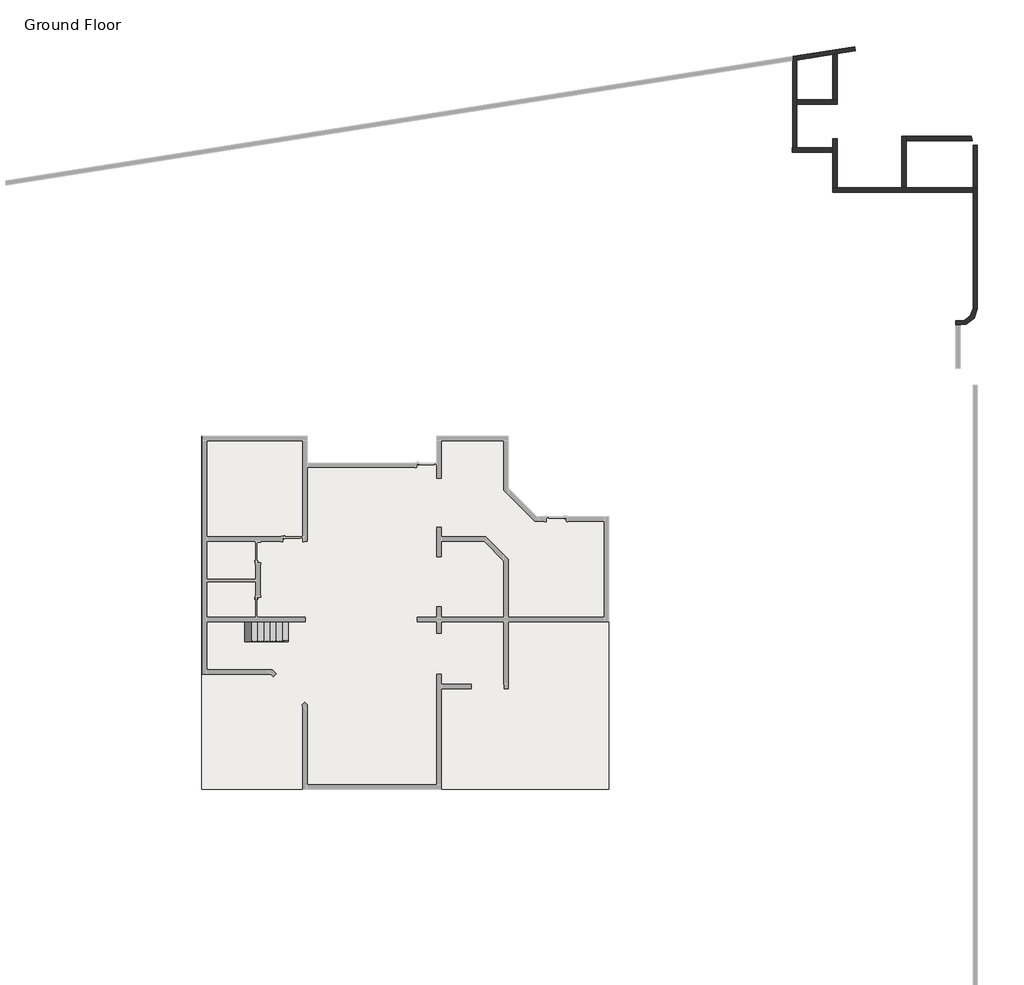
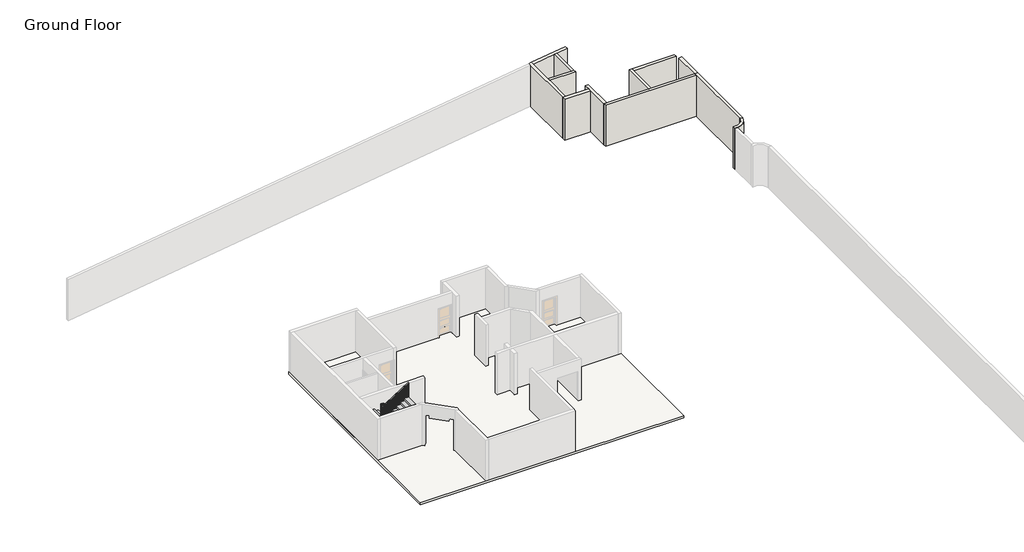
# One storey, part 2 of 2: 12 walls, 1 railing, 1 slab, 1 stair flight.
"""IFC4 building model written with IfcOpenShell, lengths in millimetres."""

from ifc_helpers import new_model, si_unit, point, frame, frame_2d, origin, origin_with_axes, place, context, project, spatial, polyline, circle_curve, trimmed, segment, composite_curve, outline, extrude, faceted_brep, element, save
from ifc_brep_helpers import plane_surface, cylinder_surface, revolved_surface, advanced_brep

model = new_model("IFC4")

# Units and contexts
model_context = context("Model", 3, world=origin())
ifc_project = project(units=[si_unit("LENGTHUNIT", "METRE", prefix="MILLI")], contexts=[model_context])

# Site, building, storey
site = spatial("IfcSite", under=ifc_project)
building = spatial("IfcBuilding", under=site)
storey = spatial("IfcBuildingStorey", under=building, Name="Ground Floor", Elevation=0.0)

# Railing
placement = place(None, origin())
element("IfcRailing", 1, ObjectType="Handrail - Rectangular", at=placement, inside=storey, context=model_context, shape_type="SolidModel", body=[
    faceted_brep([(-22136.7199287, -1918.1666371, 1093.6941176), (-22136.7199287, -1918.1666371, 1033.3090189), (-22136.7199287, -1867.3666371, 1033.3090189), (-22136.7199287, -1867.3666371, 1093.6941176), (-24850.5453762, -1918.1666371, 2837.6672398), (-24901.3453762, -1918.1666371, 2809.9275106), (-24901.3453762, -1867.3666371, 2809.9275106), (-24850.5453762, -1867.3666371, 2837.6672398), (-24926.7453762, -1994.3666371, 2835.8352941), (-24926.7453762, -1994.3666371, 2886.6352941), (-24926.7453762, -2196.4192808, 2886.6352941), (-24926.7453762, -2247.2192808, 2835.8352941), (-24977.5453762, -1994.3666371, 2835.8352941), (-24977.5453762, -2247.2192808, 2835.8352941), (-24977.5453762, -1994.3666371, 2886.6352941), (-24977.5453762, -2196.4192808, 2886.6352941), (-23259.8703762, -2272.6192808, 4141.6941176), (-23259.8703762, -2323.4192808, 4141.6941176), (-23259.8703762, -2323.4192808, 4081.2333039), (-23259.8703762, -2272.6192808, 4081.2333039), (-24835.5761466, -2272.6192808, 3064.3072269), (-24850.5453762, -2272.6192808, 3115.1072269), (-24835.5761466, -2323.4192808, 3064.3072269), (-24850.5453762, -2323.4192808, 3115.1072269), (-24850.5453762, -1918.1666371, 2886.6352941), (-24901.3453762, -1918.1666371, 2835.8352941), (-24901.3453762, -1867.3666371, 2835.8352941), (-24850.5453762, -1867.3666371, 2886.6352941), (-24926.7453762, -1918.1666371, 2886.6352941), (-24926.7453762, -1918.1666371, 2835.8352941), (-24977.5453762, -1867.3666371, 2835.8352941), (-24977.5453762, -1867.3666371, 2886.6352941), (-24926.7453762, -2196.4192808, 3115.1072269), (-24926.7453762, -2247.2192808, 3064.3072269), (-24977.5453762, -2247.2192808, 3064.3072269), (-24977.5453762, -2196.4192808, 3115.1072269), (-24926.7453762, -2272.6192808, 3115.1072269), (-24926.7453762, -2272.6192808, 3064.3072269), (-24977.5453762, -2323.4192808, 3064.3072269), (-24977.5453762, -2323.4192808, 3115.1072269)], [[[0, 1, 2, 3]], [[1, 0, 4, 5]], [[2, 1, 5, 6]], [[3, 2, 6, 7]], [[0, 3, 7, 4]], [[8, 9, 10, 11]], [[12, 8, 11, 13]], [[14, 12, 13, 15]], [[9, 14, 15, 10]], [[16, 17, 18, 19]], [[20, 21, 16, 19]], [[22, 20, 19, 18]], [[23, 22, 18, 17]], [[21, 23, 17, 16]], [[5, 4, 24, 25]], [[6, 5, 25, 26]], [[7, 6, 26, 27]], [[4, 7, 27, 24]], [[25, 24, 28, 29]], [[26, 25, 29, 30]], [[27, 26, 30, 31]], [[24, 27, 31, 28]], [[29, 28, 9, 8]], [[30, 29, 8, 12]], [[31, 30, 12, 14]], [[28, 31, 14, 9]], [[11, 10, 32, 33]], [[13, 11, 33, 34]], [[15, 13, 34, 35]], [[10, 15, 35, 32]], [[33, 32, 36, 37]], [[34, 33, 37, 38]], [[35, 34, 38, 39]], [[32, 35, 39, 36]], [[37, 36, 21, 20]], [[38, 37, 20, 22]], [[39, 38, 22, 23]], [[36, 39, 23, 21]]]),
    extrude(outline(polyline([(4032.0554888, -23336.0703762), (3048.0, -23336.0703762), (3048.0, -23317.0203762), (4044.3499425, -23317.0203762), (4032.0554888, -23336.0703762)])), frame((0.0, -2307.5442808, 0.0), z_axis=(0.0, 1.0, 0.0), x_axis=(0.0, 0.0, 1.0)), (0.0, 0.0, 1.0), 19.05),
    extrude(outline(polyline([(3966.4850686, -23437.6703762), (3048.0, -23437.6703762), (3048.0, -23418.6203762), (3978.7795224, -23418.6203762), (3966.4850686, -23437.6703762)])), frame((0.0, -2307.5442808, 0.0), z_axis=(0.0, 1.0, 0.0), x_axis=(0.0, 0.0, 1.0)), (0.0, 0.0, 1.0), 19.05),
    extrude(outline(polyline([(3900.9146484, -23539.2703762), (3048.0, -23539.2703762), (3048.0, -23520.2203762), (3913.2091022, -23520.2203762), (3900.9146484, -23539.2703762)])), frame((0.0, -2307.5442808, 0.0), z_axis=(0.0, 1.0, 0.0), x_axis=(0.0, 0.0, 1.0)), (0.0, 0.0, 1.0), 19.05),
    extrude(outline(polyline([(3835.3442283, -23640.8703762), (2868.7058824, -23640.8703762), (2868.7058824, -23621.8203762), (3847.638682, -23621.8203762), (3835.3442283, -23640.8703762)])), frame((0.0, -2307.5442808, 0.0), z_axis=(0.0, 1.0, 0.0), x_axis=(0.0, 0.0, 1.0)), (0.0, 0.0, 1.0), 19.05),
    extrude(outline(polyline([(3769.7738081, -23742.4703762), (2868.7058824, -23742.4703762), (2868.7058824, -23723.4203762), (3782.0682619, -23723.4203762), (3769.7738081, -23742.4703762)])), frame((0.0, -2307.5442808, 0.0), z_axis=(0.0, 1.0, 0.0), x_axis=(0.0, 0.0, 1.0)), (0.0, 0.0, 1.0), 19.05),
    extrude(outline(polyline([(3704.2033879, -23844.0703762), (2689.4117647, -23844.0703762), (2689.4117647, -23825.0203762), (3716.4978417, -23825.0203762), (3704.2033879, -23844.0703762)])), frame((0.0, -2307.5442808, 0.0), z_axis=(0.0, 1.0, 0.0), x_axis=(0.0, 0.0, 1.0)), (0.0, 0.0, 1.0), 19.05),
    extrude(outline(polyline([(3638.6329678, -23945.6703762), (2689.4117647, -23945.6703762), (2689.4117647, -23926.6203762), (3650.9274215, -23926.6203762), (3638.6329678, -23945.6703762)])), frame((0.0, -2307.5442808, 0.0), z_axis=(0.0, 1.0, 0.0), x_axis=(0.0, 0.0, 1.0)), (0.0, 0.0, 1.0), 19.05),
    extrude(outline(polyline([(3573.0625476, -24047.2703762), (2689.4117647, -24047.2703762), (2689.4117647, -24028.2203762), (3585.3570014, -24028.2203762), (3573.0625476, -24047.2703762)])), frame((0.0, -2307.5442808, 0.0), z_axis=(0.0, 1.0, 0.0), x_axis=(0.0, 0.0, 1.0)), (0.0, 0.0, 1.0), 19.05),
    extrude(outline(polyline([(3507.4921274, -24148.8703762), (2510.1176471, -24148.8703762), (2510.1176471, -24129.8203762), (3519.7865812, -24129.8203762), (3507.4921274, -24148.8703762)])), frame((0.0, -2307.5442808, 0.0), z_axis=(0.0, 1.0, 0.0), x_axis=(0.0, 0.0, 1.0)), (0.0, 0.0, 1.0), 19.05),
    extrude(outline(polyline([(3441.9236988, -24250.4703762), (2510.1176471, -24250.4703762), (2510.1176471, -24231.4203762), (3454.1657124, -24231.4203762), (3441.9236988, -24250.4703762)])), frame((0.0, -2307.5442808, 0.0), z_axis=(0.0, 1.0, 0.0), x_axis=(0.0, 0.0, 1.0)), (0.0, 0.0, 1.0), 19.05),
    extrude(outline(polyline([(3376.3512871, -24352.0703762), (2510.1176471, -24352.0703762), (2510.1176471, -24333.0203762), (3388.6457409, -24333.0203762), (3376.3512871, -24352.0703762)])), frame((0.0, -2307.5442808, 0.0), z_axis=(0.0, 1.0, 0.0), x_axis=(0.0, 0.0, 1.0)), (0.0, 0.0, 1.0), 19.05),
    extrude(outline(polyline([(3310.7808669, -24453.6703762), (2330.8235294, -24453.6703762), (2330.8235294, -24434.6203762), (3323.0753207, -24434.6203762), (3310.7808669, -24453.6703762)])), frame((0.0, -2307.5442808, 0.0), z_axis=(0.0, 1.0, 0.0), x_axis=(0.0, 0.0, 1.0)), (0.0, 0.0, 1.0), 19.05),
    extrude(outline(polyline([(3245.2104467, -24555.2703762), (2330.8235294, -24555.2703762), (2330.8235294, -24536.2203762), (3257.5049005, -24536.2203762), (3245.2104467, -24555.2703762)])), frame((0.0, -2307.5442808, 0.0), z_axis=(0.0, 1.0, 0.0), x_axis=(0.0, 0.0, 1.0)), (0.0, 0.0, 1.0), 19.05),
    extrude(outline(polyline([(3179.6400266, -24656.8703762), (2330.8235294, -24656.8703762), (2330.8235294, -24637.8203762), (3191.9344804, -24637.8203762), (3179.6400266, -24656.8703762)])), frame((0.0, -2307.5442808, 0.0), z_axis=(0.0, 1.0, 0.0), x_axis=(0.0, 0.0, 1.0)), (0.0, 0.0, 1.0), 19.05),
    extrude(outline(polyline([(3114.0696064, -24758.4703762), (2151.5294118, -24758.4703762), (2151.5294118, -24739.4203762), (3126.3640602, -24739.4203762), (3114.0696064, -24758.4703762)])), frame((0.0, -2307.5442808, 0.0), z_axis=(0.0, 1.0, 0.0), x_axis=(0.0, 0.0, 1.0)), (0.0, 0.0, 1.0), 19.05),
    extrude(outline(polyline([(3048.4991862, -24860.0703762), (2151.5294118, -24860.0703762), (2151.5294118, -24841.0203762), (3060.79364, -24841.0203762), (3048.4991862, -24860.0703762)])), frame((0.0, -2307.5442808, 0.0), z_axis=(0.0, 1.0, 0.0), x_axis=(0.0, 0.0, 1.0)), (0.0, 0.0, 1.0), 19.05),
    extrude(outline(polyline([(-24942.6203762, -2188.0416371), (-24942.6203762, -2207.0916371), (-24961.6703762, -2207.0916371), (-24961.6703762, -2188.0416371), (-24942.6203762, -2188.0416371)])), frame((0.0, 0.0, 1972.2352941), z_axis=(0.0, 0.0, 1.0), x_axis=(1.0, 0.0, 0.0)), (0.0, 0.0, 1.0), 1092.0719328),
    extrude(outline(polyline([(-24942.6203762, -2086.4416371), (-24942.6203762, -2105.4916371), (-24961.6703762, -2105.4916371), (-24961.6703762, -2086.4416371), (-24942.6203762, -2086.4416371)])), frame((0.0, 0.0, 1972.2352941), z_axis=(0.0, 0.0, 1.0), x_axis=(1.0, 0.0, 0.0)), (0.0, 0.0, 1.0), 863.6),
    extrude(outline(polyline([(-24942.6203762, -1984.8416371), (-24942.6203762, -2003.8916371), (-24961.6703762, -2003.8916371), (-24961.6703762, -1984.8416371), (-24942.6203762, -1984.8416371)])), frame((0.0, 0.0, 1972.2352941), z_axis=(0.0, 0.0, 1.0), x_axis=(1.0, 0.0, 0.0)), (0.0, 0.0, 1.0), 863.6),
    extrude(outline(polyline([(-24870.3949287, -1902.2916371), (-24889.4449287, -1902.2916371), (-24889.4449287, -1883.2416371), (-24870.3949287, -1883.2416371), (-24870.3949287, -1902.2916371)])), frame((0.0, 0.0, 1792.9411765), z_axis=(0.0, 0.0, 1.0), x_axis=(1.0, 0.0, 0.0)), (0.0, 0.0, 1.0), 1042.8941176),
    extrude(outline(polyline([(2736.9892418, -24787.8449287), (1792.9411765, -24787.8449287), (1792.9411765, -24768.7949287), (2724.7472283, -24768.7949287), (2736.9892418, -24787.8449287)])), frame((0.0, -1902.2916371, 0.0), z_axis=(0.0, 1.0, 0.0), x_axis=(0.0, 0.0, 1.0)), (0.0, 0.0, 1.0), 19.05),
    extrude(outline(polyline([(2671.6985028, -24686.2449287), (1792.9411765, -24686.2449287), (1792.9411765, -24667.1949287), (2659.4564892, -24667.1949287), (2671.6985028, -24686.2449287)])), frame((0.0, -1902.2916371, 0.0), z_axis=(0.0, 1.0, 0.0), x_axis=(0.0, 0.0, 1.0)), (0.0, 0.0, 1.0), 19.05),
    extrude(outline(polyline([(2606.4077637, -24584.6449287), (1613.6470588, -24584.6449287), (1613.6470588, -24565.5949287), (2594.1657501, -24565.5949287), (2606.4077637, -24584.6449287)])), frame((0.0, -1902.2916371, 0.0), z_axis=(0.0, 1.0, 0.0), x_axis=(0.0, 0.0, 1.0)), (0.0, 0.0, 1.0), 19.05),
    extrude(outline(polyline([(2541.1170246, -24483.0449287), (1613.6470588, -24483.0449287), (1613.6470588, -24463.9949287), (2528.875011, -24463.9949287), (2541.1170246, -24483.0449287)])), frame((0.0, -1902.2916371, 0.0), z_axis=(0.0, 1.0, 0.0), x_axis=(0.0, 0.0, 1.0)), (0.0, 0.0, 1.0), 19.05),
    extrude(outline(polyline([(2475.8262855, -24381.4449287), (1613.6470588, -24381.4449287), (1613.6470588, -24362.3949287), (2463.5842719, -24362.3949287), (2475.8262855, -24381.4449287)])), frame((0.0, -1902.2916371, 0.0), z_axis=(0.0, 1.0, 0.0), x_axis=(0.0, 0.0, 1.0)), (0.0, 0.0, 1.0), 19.05),
    extrude(outline(polyline([(2410.5355464, -24279.8449287), (1434.3529412, -24279.8449287), (1434.3529412, -24260.7949287), (2398.2935328, -24260.7949287), (2410.5355464, -24279.8449287)])), frame((0.0, -1902.2916371, 0.0), z_axis=(0.0, 1.0, 0.0), x_axis=(0.0, 0.0, 1.0)), (0.0, 0.0, 1.0), 19.05),
    extrude(outline(polyline([(2345.2448073, -24178.2449287), (1434.3529412, -24178.2449287), (1434.3529412, -24159.1949287), (2333.0027938, -24159.1949287), (2345.2448073, -24178.2449287)])), frame((0.0, -1902.2916371, 0.0), z_axis=(0.0, 1.0, 0.0), x_axis=(0.0, 0.0, 1.0)), (0.0, 0.0, 1.0), 19.05),
    extrude(outline(polyline([(2279.9540683, -24076.6449287), (1255.0588235, -24076.6449287), (1255.0588235, -24057.5949287), (2267.7120547, -24057.5949287), (2279.9540683, -24076.6449287)])), frame((0.0, -1902.2916371, 0.0), z_axis=(0.0, 1.0, 0.0), x_axis=(0.0, 0.0, 1.0)), (0.0, 0.0, 1.0), 19.05),
    extrude(outline(polyline([(2214.6633292, -23975.0449287), (1255.0588235, -23975.0449287), (1255.0588235, -23955.9949287), (2202.4213156, -23955.9949287), (2214.6633292, -23975.0449287)])), frame((0.0, -1902.2916371, 0.0), z_axis=(0.0, 1.0, 0.0), x_axis=(0.0, 0.0, 1.0)), (0.0, 0.0, 1.0), 19.05),
    extrude(outline(polyline([(2149.3725901, -23873.4449287), (1255.0588235, -23873.4449287), (1255.0588235, -23854.3949287), (2137.1305765, -23854.3949287), (2149.3725901, -23873.4449287)])), frame((0.0, -1902.2916371, 0.0), z_axis=(0.0, 1.0, 0.0), x_axis=(0.0, 0.0, 1.0)), (0.0, 0.0, 1.0), 19.05),
    extrude(outline(polyline([(2084.081851, -23771.8449287), (1075.7647059, -23771.8449287), (1075.7647059, -23752.7949287), (2071.8398374, -23752.7949287), (2084.081851, -23771.8449287)])), frame((0.0, -1902.2916371, 0.0), z_axis=(0.0, 1.0, 0.0), x_axis=(0.0, 0.0, 1.0)), (0.0, 0.0, 1.0), 19.05),
    extrude(outline(polyline([(2018.7911119, -23670.2449287), (1075.7647059, -23670.2449287), (1075.7647059, -23651.1949287), (2006.5490983, -23651.1949287), (2018.7911119, -23670.2449287)])), frame((0.0, -1902.2916371, 0.0), z_axis=(0.0, 1.0, 0.0), x_axis=(0.0, 0.0, 1.0)), (0.0, 0.0, 1.0), 19.05),
    extrude(outline(polyline([(1953.5003728, -23568.6449287), (1075.7647059, -23568.6449287), (1075.7647059, -23549.5949287), (1941.2583593, -23549.5949287), (1953.5003728, -23568.6449287)])), frame((0.0, -1902.2916371, 0.0), z_axis=(0.0, 1.0, 0.0), x_axis=(0.0, 0.0, 1.0)), (0.0, 0.0, 1.0), 19.05),
    extrude(outline(polyline([(1888.2096338, -23467.0449287), (896.4705882, -23467.0449287), (896.4705882, -23447.9949287), (1875.9676202, -23447.9949287), (1888.2096338, -23467.0449287)])), frame((0.0, -1902.2916371, 0.0), z_axis=(0.0, 1.0, 0.0), x_axis=(0.0, 0.0, 1.0)), (0.0, 0.0, 1.0), 19.05),
    extrude(outline(polyline([(1822.9188947, -23365.4449287), (896.4705882, -23365.4449287), (896.4705882, -23346.3949287), (1810.6768811, -23346.3949287), (1822.9188947, -23365.4449287)])), frame((0.0, -1902.2916371, 0.0), z_axis=(0.0, 1.0, 0.0), x_axis=(0.0, 0.0, 1.0)), (0.0, 0.0, 1.0), 19.05),
    extrude(outline(polyline([(1757.6281556, -23263.8449287), (717.1764706, -23263.8449287), (717.1764706, -23244.7949287), (1745.386142, -23244.7949287), (1757.6281556, -23263.8449287)])), frame((0.0, -1902.2916371, 0.0), z_axis=(0.0, 1.0, 0.0), x_axis=(0.0, 0.0, 1.0)), (0.0, 0.0, 1.0), 19.05),
    extrude(outline(polyline([(1692.3374165, -23162.2449287), (717.1764706, -23162.2449287), (717.1764706, -23143.1949287), (1680.0954029, -23143.1949287), (1692.3374165, -23162.2449287)])), frame((0.0, -1902.2916371, 0.0), z_axis=(0.0, 1.0, 0.0), x_axis=(0.0, 0.0, 1.0)), (0.0, 0.0, 1.0), 19.05),
    extrude(outline(polyline([(1627.0466774, -23060.6449287), (717.1764706, -23060.6449287), (717.1764706, -23041.5949287), (1614.8046638, -23041.5949287), (1627.0466774, -23060.6449287)])), frame((0.0, -1902.2916371, 0.0), z_axis=(0.0, 1.0, 0.0), x_axis=(0.0, 0.0, 1.0)), (0.0, 0.0, 1.0), 19.05),
    extrude(outline(polyline([(1561.7559383, -22959.0449287), (537.8823529, -22959.0449287), (537.8823529, -22939.9949287), (1549.5139248, -22939.9949287), (1561.7559383, -22959.0449287)])), frame((0.0, -1902.2916371, 0.0), z_axis=(0.0, 1.0, 0.0), x_axis=(0.0, 0.0, 1.0)), (0.0, 0.0, 1.0), 19.05),
    extrude(outline(polyline([(1496.4651993, -22857.4449287), (537.8823529, -22857.4449287), (537.8823529, -22838.3949287), (1484.2231857, -22838.3949287), (1496.4651993, -22857.4449287)])), frame((0.0, -1902.2916371, 0.0), z_axis=(0.0, 1.0, 0.0), x_axis=(0.0, 0.0, 1.0)), (0.0, 0.0, 1.0), 19.05),
    extrude(outline(polyline([(1431.1744602, -22755.8449287), (537.8823529, -22755.8449287), (537.8823529, -22736.7949287), (1418.9324466, -22736.7949287), (1431.1744602, -22755.8449287)])), frame((0.0, -1902.2916371, 0.0), z_axis=(0.0, 1.0, 0.0), x_axis=(0.0, 0.0, 1.0)), (0.0, 0.0, 1.0), 19.05),
    extrude(outline(polyline([(1365.8837211, -22654.2449287), (358.5882353, -22654.2449287), (358.5882353, -22635.1949287), (1353.6417075, -22635.1949287), (1365.8837211, -22654.2449287)])), frame((0.0, -1902.2916371, 0.0), z_axis=(0.0, 1.0, 0.0), x_axis=(0.0, 0.0, 1.0)), (0.0, 0.0, 1.0), 19.05),
    extrude(outline(polyline([(1300.592982, -22552.6449287), (358.5882353, -22552.6449287), (358.5882353, -22533.5949287), (1288.3509684, -22533.5949287), (1300.592982, -22552.6449287)])), frame((0.0, -1902.2916371, 0.0), z_axis=(0.0, 1.0, 0.0), x_axis=(0.0, 0.0, 1.0)), (0.0, 0.0, 1.0), 19.05),
    extrude(outline(polyline([(1235.3022429, -22451.0449287), (358.5882353, -22451.0449287), (358.5882353, -22431.9949287), (1223.0602293, -22431.9949287), (1235.3022429, -22451.0449287)])), frame((0.0, -1902.2916371, 0.0), z_axis=(0.0, 1.0, 0.0), x_axis=(0.0, 0.0, 1.0)), (0.0, 0.0, 1.0), 19.05),
    extrude(outline(polyline([(1170.0115038, -22349.4449287), (179.2941176, -22349.4449287), (179.2941176, -22330.3949287), (1157.7694903, -22330.3949287), (1170.0115038, -22349.4449287)])), frame((0.0, -1902.2916371, 0.0), z_axis=(0.0, 1.0, 0.0), x_axis=(0.0, 0.0, 1.0)), (0.0, 0.0, 1.0), 19.05),
    extrude(outline(polyline([(1104.7207648, -22247.8449287), (179.2941176, -22247.8449287), (179.2941176, -22228.7949287), (1092.4787512, -22228.7949287), (1104.7207648, -22247.8449287)])), frame((0.0, -1902.2916371, 0.0), z_axis=(0.0, 1.0, 0.0), x_axis=(0.0, 0.0, 1.0)), (0.0, 0.0, 1.0), 19.05),
    extrude(outline(polyline([(-24942.6203762, -2288.4942808), (-24942.6203762, -2307.5442808), (-24961.6703762, -2307.5442808), (-24961.6703762, -2288.4942808), (-24942.6203762, -2288.4942808)])), frame((0.0, 0.0, 1972.2352941), z_axis=(0.0, 0.0, 1.0), x_axis=(1.0, 0.0, 0.0)), (0.0, 0.0, 1.0), 1092.0719328),
    extrude(outline(polyline([(-24942.6203762, -1902.2916371), (-24961.6703762, -1902.2916371), (-24961.6703762, -1883.2416371), (-24942.6203762, -1883.2416371), (-24942.6203762, -1902.2916371)])), frame((0.0, 0.0, 1972.2352941), z_axis=(0.0, 0.0, 1.0), x_axis=(1.0, 0.0, 0.0)), (0.0, 0.0, 1.0), 863.6),
    extrude(outline(polyline([(4068.9388501, -23278.9203762), (3048.0, -23278.9203762), (3048.0, -23259.8703762), (4081.2333039, -23259.8703762), (4068.9388501, -23278.9203762)])), frame((0.0, -2307.5442808, 0.0), z_axis=(0.0, 1.0, 0.0), x_axis=(0.0, 0.0, 1.0)), (0.0, 0.0, 1.0), 19.05),
    extrude(outline(polyline([(1045.5510325, -22155.7699287), (179.2941176, -22155.7699287), (179.2941176, -22136.7199287), (1033.3090189, -22136.7199287), (1045.5510325, -22155.7699287)])), frame((0.0, -1902.2916371, 0.0), z_axis=(0.0, 1.0, 0.0), x_axis=(0.0, 0.0, 1.0)), (0.0, 0.0, 1.0), 19.05),
])

# Slab
element("IfcSlab", 2, ObjectType="Generic - 6\"", at=placement, inside=storey, context=model_context, shape_type="SweptSolid", body=[
    extrude(outline(polyline([(-26070.8685036, 7427.7381656), (-21270.0431154, 7427.7381656), (-21270.0431154, 6211.8276825), (-15383.4246912, 6211.8276825), (-15383.4246912, 7427.7381656), (-12133.7209731, 7427.7381656), (-12133.7209731, 5061.8092257), (-10842.9476523, 3771.0359048), (-7561.7197767, 3771.0359048), (-7561.7197767, -8625.8614616), (-26070.8685036, -8625.8614616), (-26070.8685036, 7427.7381656)])), frame((0.0, 0.0, -152.4), z_axis=(0.0, 0.0, 1.0), x_axis=(1.0, 0.0, 0.0)), (0.0, 0.0, 1.0), 152.4),
])

# Stair flight
element("IfcStairFlight", 3, ObjectType="3/4\" Nosing", at=placement, inside=storey, context=model_context, shape_type="Brep", body=[
    faceted_brep([(-22414.5324287, -1918.1666371, 179.2941176), (-22136.7199287, -1918.1666371, 179.2941176), (-22136.7199287, -1002.5777916, 179.2941176), (-22414.5324287, -1002.5777916, 179.2941176), (-22414.5324287, -1918.1666371, 115.7941176), (-22136.7199287, -1918.1666371, 115.7941176), (-22136.7199287, -1002.5777916, 115.7941176), (-22414.5324287, -1002.5777916, 115.7941176), (-22433.1694115, -1918.1666371, 115.7941176), (-22433.1694115, -1002.5777916, 115.7941176), (-22704.2453762, -1918.1666371, 289.9118944), (-22982.0578762, -1918.1666371, 468.3566891), (-23259.8703762, -1918.1666371, 646.8014837), (-23537.6828762, -1918.1666371, 825.2462784), (-23815.4953762, -1918.1666371, 1003.691073), (-24093.3078762, -1918.1666371, 1182.1358677), (-24371.1203762, -1918.1666371, 1360.5806623), (-24648.9328762, -1918.1666371, 1539.025457), (-25224.5171309, -1918.1666371, 1908.7352941), (-25224.5171309, -1002.5777916, 1908.7352941), (-24926.7453762, -1002.5777916, 1717.4702516), (-24648.9328762, -1002.5777916, 1539.025457), (-24371.1203762, -1002.5777916, 1360.5806623), (-24093.3078762, -1002.5777916, 1182.1358677), (-23815.4953762, -1002.5777916, 1003.691073), (-23537.6828762, -1002.5777916, 825.2462784), (-23259.8703762, -1002.5777916, 646.8014837), (-22982.0578762, -1002.5777916, 468.3566891), (-22704.2453762, -1002.5777916, 289.9118944), (-24926.7453762, -1918.1666371, 1908.7352941), (-24926.7453762, -2272.6192808, 1908.7352941), (-24908.0338391, -2272.6192808, 1908.7352941), (-24908.0338391, -3187.915973, 1908.7352941), (-24926.7453762, -3187.915973, 1908.7352941), (-25842.0443119, -3187.915973, 1908.7352941), (-25842.0443119, -1002.5777916, 1908.7352941), (-24648.9328762, -2272.6192808, 2075.9533946), (-24371.1203762, -2272.6192808, 2255.2475122), (-24093.3078762, -2272.6192808, 2434.5416299), (-23815.4953762, -2272.6192808, 2613.8357475), (-23537.6828762, -2272.6192808, 2793.1298652), (-23259.8703762, -2272.6192808, 2972.4239828), (-23259.8703762, -3187.915973, 2972.4239828), (-23537.6828762, -3187.915973, 2793.1298652), (-23815.4953762, -3187.915973, 2613.8357475), (-24093.3078762, -3187.915973, 2434.5416299), (-24371.1203762, -3187.915973, 2255.2475122), (-24648.9328762, -3187.915973, 2075.9533946), (-22414.5324287, -1918.1666371, 358.5882353), (-22414.5324287, -1002.5777916, 358.5882353), (-22433.1694115, -1002.5777916, 358.5882353), (-22704.2453762, -1002.5777916, 358.5882353), (-22704.2453762, -1918.1666371, 358.5882353), (-22433.1694115, -1918.1666371, 358.5882353), (-22982.0578762, -1918.1666371, 537.8823529), (-22704.2453762, -1918.1666371, 537.8823529), (-22704.2453762, -1002.5777916, 537.8823529), (-22982.0578762, -1002.5777916, 537.8823529), (-23259.8703762, -1918.1666371, 717.1764706), (-22982.0578762, -1918.1666371, 717.1764706), (-22982.0578762, -1002.5777916, 717.1764706), (-23259.8703762, -1002.5777916, 717.1764706), (-23537.6828762, -1918.1666371, 896.4705882), (-23259.8703762, -1918.1666371, 896.4705882), (-23259.8703762, -1002.5777916, 896.4705882), (-23537.6828762, -1002.5777916, 896.4705882), (-23815.4953762, -1918.1666371, 1075.7647059), (-23537.6828762, -1918.1666371, 1075.7647059), (-23537.6828762, -1002.5777916, 1075.7647059), (-23815.4953762, -1002.5777916, 1075.7647059), (-24093.3078762, -1918.1666371, 1255.0588235), (-23815.4953762, -1918.1666371, 1255.0588235), (-23815.4953762, -1002.5777916, 1255.0588235), (-24093.3078762, -1002.5777916, 1255.0588235), (-24371.1203762, -1918.1666371, 1434.3529412), (-24093.3078762, -1918.1666371, 1434.3529412), (-24093.3078762, -1002.5777916, 1434.3529412), (-24371.1203762, -1002.5777916, 1434.3529412), (-24648.9328762, -1918.1666371, 1613.6470588), (-24371.1203762, -1918.1666371, 1613.6470588), (-24371.1203762, -1002.5777916, 1613.6470588), (-24648.9328762, -1002.5777916, 1613.6470588), (-24926.7453762, -1918.1666371, 1792.9411765), (-24648.9328762, -1918.1666371, 1792.9411765), (-24648.9328762, -1002.5777916, 1792.9411765), (-24926.7453762, -1002.5777916, 1792.9411765), (-24926.7453762, -2272.6192808, 1972.2352941), (-24926.7453762, -1918.1666371, 1972.2352941), (-24926.7453762, -1002.5777916, 1972.2352941), (-25224.5171309, -1002.5777916, 1972.2352941), (-25842.0443119, -1002.5777916, 1972.2352941), (-25842.0443119, -3187.915973, 1972.2352941), (-24926.7453762, -3187.915973, 1972.2352941), (-24926.7453762, -2272.6192808, 2151.5294118), (-24926.7453762, -3187.915973, 2151.5294118), (-24908.0338391, -3187.915973, 2151.5294118), (-24648.9328762, -3187.915973, 2151.5294118), (-24648.9328762, -2272.6192808, 2151.5294118), (-24908.0338391, -2272.6192808, 2151.5294118), (-24371.1203762, -2272.6192808, 2330.8235294), (-24648.9328762, -2272.6192808, 2330.8235294), (-24648.9328762, -3187.915973, 2330.8235294), (-24371.1203762, -3187.915973, 2330.8235294), (-24093.3078762, -2272.6192808, 2510.1176471), (-24371.1203762, -2272.6192808, 2510.1176471), (-24371.1203762, -3187.915973, 2510.1176471), (-24093.3078762, -3187.915973, 2510.1176471), (-23815.4953762, -2272.6192808, 2689.4117647), (-24093.3078762, -2272.6192808, 2689.4117647), (-24093.3078762, -3187.915973, 2689.4117647), (-23815.4953762, -3187.915973, 2689.4117647), (-23537.6828762, -2272.6192808, 2868.7058824), (-23815.4953762, -2272.6192808, 2868.7058824), (-23815.4953762, -3187.915973, 2868.7058824), (-23537.6828762, -3187.915973, 2868.7058824), (-23259.8703762, -2272.6192808, 3048.0), (-23537.6828762, -2272.6192808, 3048.0), (-23537.6828762, -3187.915973, 3048.0), (-23259.8703762, -3187.915973, 3048.0)], [[[0, 1, 2, 3]], [[1, 0, 4, 5]], [[2, 1, 5, 6]], [[3, 2, 6, 7]], [[8, 9, 7, 6, 5, 4]], [[9, 8, 10, 11, 12, 13, 14, 15, 16, 17, 18, 19, 20, 21, 22, 23, 24, 25, 26, 27, 28]], [[19, 18, 29, 30, 31, 32, 33, 34, 35]], [[32, 31, 36, 37, 38, 39, 40, 41, 42, 43, 44, 45, 46, 47]], [[48, 49, 50, 51, 52, 53]], [[0, 48, 53, 52, 10, 8, 4]], [[0, 3, 49, 48]], [[49, 3, 7, 9, 28, 51, 50]], [[54, 55, 56, 57]], [[55, 54, 11, 10, 52]], [[52, 51, 56, 55]], [[57, 56, 51, 28, 27]], [[58, 59, 60, 61]], [[59, 58, 12, 11, 54]], [[54, 57, 60, 59]], [[61, 60, 57, 27, 26]], [[62, 63, 64, 65]], [[63, 62, 13, 12, 58]], [[58, 61, 64, 63]], [[65, 64, 61, 26, 25]], [[66, 67, 68, 69]], [[67, 66, 14, 13, 62]], [[62, 65, 68, 67]], [[69, 68, 65, 25, 24]], [[70, 71, 72, 73]], [[71, 70, 15, 14, 66]], [[66, 69, 72, 71]], [[73, 72, 69, 24, 23]], [[74, 75, 76, 77]], [[75, 74, 16, 15, 70]], [[70, 73, 76, 75]], [[77, 76, 73, 23, 22]], [[78, 79, 80, 81]], [[79, 78, 17, 16, 74]], [[74, 77, 80, 79]], [[81, 80, 77, 22, 21]], [[82, 83, 84, 85]], [[83, 82, 29, 18, 17, 78]], [[78, 81, 84, 83]], [[85, 84, 81, 21, 20]], [[86, 87, 88, 89, 90, 91, 92]], [[87, 86, 30, 29]], [[82, 85, 88, 87, 29]], [[88, 85, 20, 19, 35, 90, 89]], [[91, 90, 35, 34]], [[92, 91, 34, 33]], [[93, 94, 95, 96, 97, 98]], [[86, 93, 98, 97, 36, 31, 30]], [[86, 92, 94, 93]], [[94, 92, 33, 32, 47, 96, 95]], [[99, 100, 101, 102]], [[100, 99, 37, 36, 97]], [[97, 96, 101, 100]], [[102, 101, 96, 47, 46]], [[103, 104, 105, 106]], [[104, 103, 38, 37, 99]], [[99, 102, 105, 104]], [[106, 105, 102, 46, 45]], [[107, 108, 109, 110]], [[108, 107, 39, 38, 103]], [[103, 106, 109, 108]], [[110, 109, 106, 45, 44]], [[111, 112, 113, 114]], [[112, 111, 40, 39, 107]], [[107, 110, 113, 112]], [[114, 113, 110, 44, 43]], [[115, 116, 117, 118]], [[116, 115, 41, 40, 111]], [[111, 114, 117, 116]], [[118, 117, 114, 43, 42]], [[115, 118, 42, 41]]]),
])

# Walls
element("IfcWall", 4, ObjectType="Generic - 0' - 7 15/16\"", at=placement, inside=storey, context=model_context, shape_type="Brep", body=[
    faceted_brep([(988.7327427, 20547.0005512, 0.0), (988.7327427, 22521.1714887, 0.0), (988.7327427, 22722.7839887, 0.0), (988.7327427, 24526.7494644, 0.0), (988.7327427, 24730.8459766, 0.0), (988.7327427, 24730.8459766, 3048.0), (988.7327427, 24526.7494644, 3048.0), (988.7327427, 22722.7839887, 3048.0), (988.7327427, 22521.1714887, 3048.0), (988.7327427, 20547.0005512, 3048.0), (787.1202427, 20547.0005512, 0.0), (787.1202427, 20547.0005512, 3048.0), (787.1202427, 24497.6518108, 3048.0), (787.1202427, 24699.1003289, 3048.0), (787.1202427, 24699.1003289, 0.0), (787.1202427, 24497.6518108, 0.0)], [[[0, 1, 2, 3, 4, 5, 6, 7, 8, 9]], [[10, 11, 12, 13, 14, 15]], [[4, 3, 2, 1, 0, 10, 15, 14]], [[9, 8, 7, 6, 5, 13, 12, 11]], [[0, 9, 11, 10]], [[5, 4, 14, 13]]]),
])
element("IfcWall", 5, ObjectType="Generic - 0' - 7 15/16\"", at=placement, inside=storey, context=model_context, shape_type="SweptSolid", body=[
    extrude(outline(polyline([(2612.9347223, 22722.7839887), (2612.9347223, 24782.4942417), (2814.5472223, 24814.2398894), (2814.5472223, 22722.7839887), (2612.9347223, 22722.7839887)])), origin_with_axes(), (0.0, 0.0, 1.0), 3048.0),
])
element("IfcWall", 6, ObjectType="Generic - 0' - 7 15/16\"", at=placement, inside=storey, context=model_context, shape_type="Brep", body=[
    faceted_brep([(988.7327427, 22521.1714887, 0.0), (2814.8394503, 22521.1714887, 0.0), (2814.8394503, 22521.1714887, 3048.0), (988.7327427, 22521.1714887, 3048.0), (988.7327427, 22722.7839887, 0.0), (988.7327427, 22722.7839887, 3048.0), (2612.9347223, 22722.7839887, 3048.0), (2814.5472223, 22722.7839887, 3048.0), (2814.8394503, 22722.7839887, 3048.0), (2814.8394503, 22722.7839887, 0.0), (2814.5472223, 22722.7839887, 0.0), (2612.9347223, 22722.7839887, 0.0)], [[[0, 1, 2, 3]], [[4, 5, 6, 7, 8, 9, 10, 11]], [[1, 0, 4, 11, 10, 9]], [[2, 1, 9, 8]], [[3, 2, 8, 7, 6, 5]], [[0, 3, 5, 4]]]),
])
element("IfcWall", 7, ObjectType="Generic - 0' - 7 15/16\"", at=placement, inside=storey, context=model_context, shape_type="SweptSolid", body=[
    extrude(outline(polyline([(2613.2269503, 20345.096945), (786.8280148, 20345.096945), (786.8280148, 20546.709445), (2613.2269503, 20546.709445), (2613.2269503, 20345.096945)])), origin_with_axes(), (0.0, 0.0, 1.0), 3048.0),
])
element("IfcWall", 8, ObjectType="Generic - 0' - 7 15/16\"", at=placement, inside=storey, context=model_context, shape_type="Brep", body=[
    faceted_brep([(2814.8394503, 18716.4061197, 0.0), (2814.8394503, 20959.7814916, 0.0), (2814.8394503, 20959.7814916, 3048.0), (2814.8394503, 18716.4061197, 3048.0), (2613.2269503, 18716.4061197, 0.0), (2613.2269503, 18716.4061197, 3048.0), (2613.2269503, 20345.096945, 3048.0), (2613.2269503, 20546.709445, 3048.0), (2613.2269503, 20959.7814916, 3048.0), (2613.2269503, 20959.7814916, 0.0), (2613.2269503, 20546.709445, 0.0), (2613.2269503, 20345.096945, 0.0)], [[[0, 1, 2, 3]], [[4, 5, 6, 7, 8, 9, 10, 11]], [[1, 0, 4, 11, 10, 9]], [[2, 1, 9, 8]], [[3, 2, 8, 7, 6, 5]], [[0, 3, 5, 4]]]),
])
element("IfcWall", 9, ObjectType="Generic - 0' - 7 15/16\"", at=placement, inside=storey, context=model_context, shape_type="SweptSolid", body=[
    extrude(outline(polyline([(8993.3885201, 18514.5013918), (2617.4213246, 18514.5013918), (2617.4213246, 18716.1138918), (8993.3885201, 18716.1138918), (8993.3885201, 18514.5013918)])), origin_with_axes(), (0.0, 0.0, 1.0), 3048.0),
])
element("IfcWall", 10, ObjectType="Generic - 0' - 7 15/16\"", at=placement, inside=storey, context=model_context, shape_type="Brep", body=[
    faceted_brep([(5951.0791763, 18716.4061197, 0.0), (5951.0791763, 20865.5600779, 0.0), (5951.0791763, 21067.1725779, 0.0), (5951.0791763, 21067.1725779, 3048.0), (5951.0791763, 20865.5600779, 3048.0), (5951.0791763, 18716.4061197, 3048.0), (5749.4666763, 18716.4061197, 0.0), (5749.4666763, 18716.4061197, 3048.0), (5749.4666763, 21067.1725779, 3048.0), (5749.4666763, 21067.1725779, 0.0)], [[[0, 1, 2, 3, 4, 5]], [[6, 7, 8, 9]], [[2, 1, 0, 6, 9]], [[5, 4, 3, 8, 7]], [[0, 5, 7, 6]], [[3, 2, 9, 8]]]),
])
element("IfcWall", 11, ObjectType="Generic - 0' - 7 15/16\"", at=placement, inside=storey, context=model_context, shape_type="SweptSolid", body=[
    extrude(outline(composite_curve([segment(polyline([(8953.0473041, 20865.5600779), (5951.0791763, 20865.5600779), (5951.0791763, 21067.1725779), (8906.823573, 21067.1725779)]), True, "CONTINUOUS"), segment(trimmed(circle_curve(frame_2d((3928.2086313, 19819.619597)), 5132.5427595), [point((8906.823573, 21067.1725779))], [point((8953.0473041, 20865.5600779))], False, "CARTESIAN"), True, "CONTINUOUS")], self_intersect=False)), origin_with_axes(), (0.0, 0.0, 1.0), 3048.0),
])
element("IfcWall", 12, ObjectType="Generic - 0' - 7 15/16\"", at=placement, inside=storey, context=model_context, shape_type="Brep", body=[
    faceted_brep([(988.7327427, 24526.7494644, 0.0), (2612.9347223, 24782.4942417, 0.0), (2814.5472223, 24814.2398894, 0.0), (3638.510131, 24943.9800407, 0.0), (3638.510131, 24943.9800407, 3048.0), (2814.5472223, 24814.2398894, 3048.0), (2612.9347223, 24782.4942417, 3048.0), (988.7327427, 24526.7494644, 3048.0), (988.7327427, 24730.8459766, 0.0), (988.7327427, 24730.8459766, 3048.0), (3616.9914994, 25144.6882566, 3048.0), (3616.9914994, 25144.6882566, 0.0)], [[[0, 1, 2, 3, 4, 5, 6, 7]], [[8, 9, 10, 11]], [[3, 2, 1, 0, 8, 11]], [[7, 6, 5, 4, 10, 9]], [[0, 7, 9, 8]], [[4, 3, 11, 10]]]),
])
element("IfcWall", 13, ObjectType="Generic - 0' - 7 15/16\"", at=placement, inside=storey, context=model_context, shape_type="SweptSolid", body=[
    extrude(outline(polyline([(9195.0010201, 20664.6700482), (9195.0010201, 18716.4061197), (8993.3885201, 18716.4061197), (8993.3885201, 20648.4427817), (9195.0010201, 20664.6700482)])), origin_with_axes(), (0.0, 0.0, 1.0), 3048.0),
])
element("IfcWall", 14, ObjectType="Generic - 0' - 7 15/16\"", at=placement, inside=storey, context=model_context, shape_type="Brep", body=[
    faceted_brep([(9195.0010201, 13233.594908, 0.0), (9195.0010201, 18716.1138918, 0.0), (9195.0010201, 18716.1138918, 3048.0), (9195.0010201, 13233.594908, 3048.0), (8993.3885201, 13238.5766944, 0.0), (8993.3885201, 13238.5766944, 3048.0), (8993.3885201, 18514.5013918, 3048.0), (8993.3885201, 18716.1138918, 3048.0), (8993.3885201, 18716.1138918, 0.0), (8993.3885201, 18514.5013918, 0.0)], [[[0, 1, 2, 3]], [[4, 5, 6, 7, 8, 9]], [[1, 0, 4, 9, 8]], [[3, 2, 7, 6, 5]], [[2, 1, 8, 7]], [[0, 3, 5, 4]]]),
])
element("IfcWall", 15, ObjectType="Generic - 0' - 7 15/16\"", at=placement, inside=storey, context=model_context, shape_type="AdvancedBrep", body=[
    advanced_brep(
    [(8993.3885201, 13238.5766944, 3048.0), (8218.7317611, 12679.9919913, 3048.0), (8218.7317611, 12472.8269263, 3048.0), (8420.3396982, 12457.4112489, 3048.0), (9195.0010201, 13233.594908, 3048.0), (8993.3885201, 13238.5766944, 0.0), (9195.0010201, 13233.594908, 0.0), (8420.3396982, 12457.4112489, 0.0), (8218.7317611, 12472.8269263, 0.0), (8218.7317611, 12679.9919913, 0.0)],
    [
        (0, 1, circle_curve(frame((8381.1692405, 13271.1676702, 3048.0), z_axis=(0.0, 0.0, -1.0), x_axis=(1.0, 0.0, 0.0)), 613.0861425)),
        (1, 2),
        (2, 3, circle_curve(frame((8381.1692405, 13271.1676702, 3048.0), z_axis=(0.0, 0.0, 1.0), x_axis=(1.0, 0.0, 0.0)), 814.6986425)),
        (3, 4, circle_curve(frame((8381.1692405, 13271.1676702, 3048.0), z_axis=(0.0, 0.0, 1.0), x_axis=(1.0, 0.0, 0.0)), 814.6986179)),
        (4, 0),
        (5, 6),
        (6, 7, circle_curve(frame((8381.1692405, 13271.1676702, 0.0), z_axis=(0.0, 0.0, -1.0), x_axis=(1.0, 0.0, 0.0)), 814.6986425)),
        (7, 8, circle_curve(frame((8381.1692405, 13271.1676702, 0.0), z_axis=(0.0, 0.0, -1.0), x_axis=(1.0, 0.0, 0.0)), 814.6986179)),
        (8, 9),
        (9, 5, circle_curve(frame((8381.1692405, 13271.1676702, 0.0), z_axis=(0.0, 0.0, 1.0), x_axis=(1.0, 0.0, 0.0)), 613.0861425)),
        (0, 5),
        (9, 1),
        (2, 8),
        (6, 4),
    ],
    [
        plane_surface(frame((8994.2553829, 13271.1676702, 3048.0), z_axis=(0.0, 0.0, 1.0), x_axis=(0.0, -1.0, 0.0))),
        plane_surface(frame((8994.2553829, 13271.1676702, 0.0), z_axis=(0.0, 0.0, -1.0), x_axis=(0.0, 1.0, 0.0))),
        revolved_surface(polyline([(8994.255383, 13271.1676702, 0.0), (8994.255383, 13271.1676702, 3048.0)]), (8381.1692405, 13271.1676702, 0.0), (0.0, 0.0, -1.0)),
        cylinder_surface(frame((8381.1692405, 13271.1676702, 0.0), z_axis=(0.0, 0.0, 1.0), x_axis=(1.0, 0.0, 0.0)), 814.6986425),
        plane_surface(frame((8218.7317611, 12658.7719349, 0.0), z_axis=(-1.0, 0.0, 0.0), x_axis=(0.0, -1.0, 0.0))),
        plane_surface(frame((9195.0010201, 13233.594908, 0.0), z_axis=(0.02470217000884842, 0.9996948548416432, 0.0), x_axis=(-0.9996948548416432, 0.02470217000884842, 0.0))),
    ],
    [
        (0, [[1, 2, 3, 4, 5]]),
        (1, [[6, 7, 8, 9, 10]]),
        (2, [[-1, 11, -10, 12]]),
        (3, [[-4, -3, 13, -8, -7, 14]]),
        (4, [[-2, -12, -9, -13]]),
        (5, [[-5, -14, -6, -11]]),
    ],
),
])

save(model, "model.ifc")

# Revit data of these elements
# Type "Handrail - Rectangular"
#   built-in parameter 1008612 = 0.0416667 (stored number, unit not read)
#   built-in parameter 1008611 = 0.0416667 (stored number, unit not read)
#   built-in parameter 1008609 = 0.333333 (stored number, unit not read)
#   built-in parameter 1008604 = 0.166667 (stored number, unit not read)
#   built-in parameter 1008603 = 0.166667 (stored number, unit not read)
#   Railing Height = 3' - 0"
#   built-in parameter 1008630 = 2
#   built-in parameter 1008610 = 2
#   built-in parameter 1008618 = Baluster - Square : 3/4"
# Type "Generic - 6\""
#   Function = 0
#   Layers, outside or top first: 0' - 6" "Concrete, Cast-in-Place gray" (function 1)
# Type "Generic - 0' - 7 15/16\""
#   Layers, outside or top first: 0' - 7 15/16" no material (function 1)
# Element 1 (IfcRailing, "Handrail - Rectangular")
#   Phase Created = New Construction
# Element 2 (IfcSlab, "Generic - 6\"")
#   built-in parameter 1001955 = 3.14159 (stored number, unit not read)
#   Height Offset From Level = 0' - 0"
#   Phase Created = New Construction
#   Materials on its faces: "Concrete, Cast-in-Place gray"
# Element 3 (IfcStairFlight, "3/4\" Nosing")
#   Phase Created = New Construction
#   Materials on its faces: "Concrete, Cast-in-Place gray"
# Elements 4, 5, 6, 7, 8, 9, 10, 11, 12, 13, 14 (IfcWall, "Generic - 0' - 7 15/16\"")
#   Top Offset = 0' - 0"
#   Base Offset = 0' - 0"
#   wall height = 10' - 0"
#   Phase Created = New Construction
#   Base Constraint = Ground Floor
#   Top Constraint = First Floor
#   Materials on its faces: "Default Wall"
# Element 15 (IfcWall, "Generic - 0' - 7 15/16\"")
#   Top Offset = 0' - 0"
#   Base Offset = 0' - 0"
#   Unconnected Height = 20' - 0"
#   wall height = 10' - 0"
#   Phase Created = New Construction
#   Materials on its faces: "Default Wall"
# Materials
#   "Concrete, Cast-in-Place gray": class "Concrete", colour RGB 192 192 192, transparency 0, Description = "Cast-in-place concrete", Cost = 0
#   "Default Wall": colour RGB 128 128 128, transparency 0, Cost = 0
